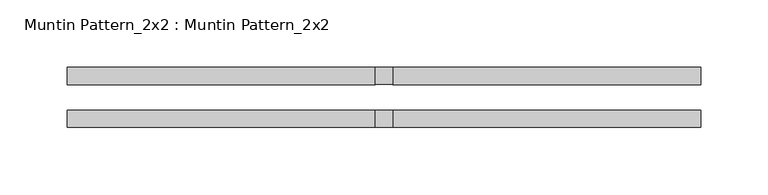
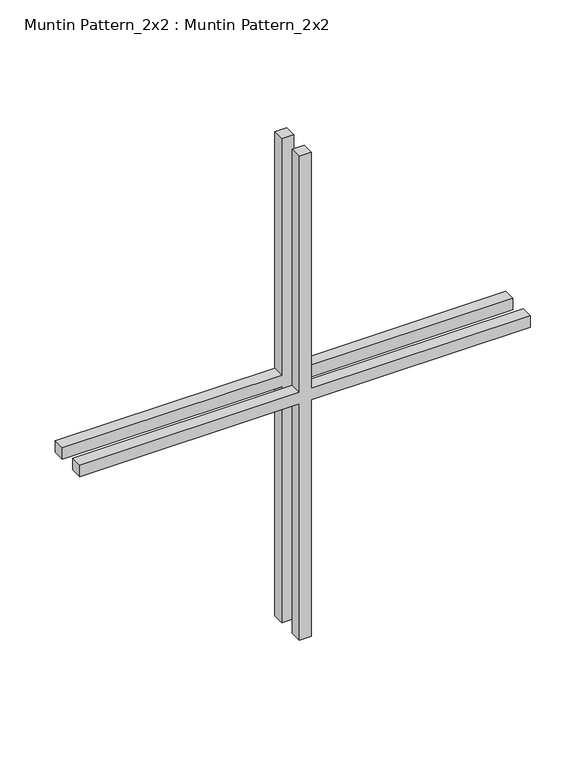
"""IFC4 building model written with IfcOpenShell, lengths in millimetres: proxy geometry, Muntin Pattern_2x2 : Muntin Pattern_2x2."""

from ifc_helpers import new_model, si_unit, frame, origin, place, context, project, spatial, polyline, outline, extrude, source, transform, mapped, element, save


def muntin_pattern_2x2_muntin_pattern_2x2_fa24e407(model_context):
    return source(origin(), model_context, "Body", "SweptSolid", [
        extrude(outline(polyline([(273.05, -6.35), (273.05, -234.95), (260.35, -234.95), (260.35, -6.35), (0.0, -6.35), (0.0, 6.35), (260.35, 6.35), (260.35, 234.95), (273.05, 234.95), (273.05, 6.35), (533.4, 6.35), (533.4, -6.35), (273.05, -6.35)])), frame((0.0, -22.225, 0.0), z_axis=(0.0, 1.0, 0.0), x_axis=(0.0, 0.0, 1.0)), (0.0, 0.0, 1.0), 12.7),
        extrude(outline(polyline([(273.05, -6.35), (273.05, -234.95), (260.35, -234.95), (260.35, -6.35), (0.0, -6.35), (0.0, 6.35), (260.35, 6.35), (260.35, 234.95), (273.05, 234.95), (273.05, 6.35), (533.4, 6.35), (533.4, -6.35), (273.05, -6.35)])), frame((0.0, 9.525, 0.0), z_axis=(0.0, 1.0, 0.0), x_axis=(0.0, 0.0, 1.0)), (0.0, 0.0, 1.0), 12.7),
    ])


if __name__ == "__main__":
    model = new_model("IFC4")
    model_context = context("Model", 3, world=origin())
    ifc_project = project(units=[si_unit("LENGTHUNIT", "METRE", prefix="MILLI")], contexts=[model_context])
    site = spatial("IfcSite", under=ifc_project)
    building = spatial("IfcBuilding", under=site)
    placement = place(None, origin())
    muntin_pattern_2x2_muntin_pattern_2x2_shape = muntin_pattern_2x2_muntin_pattern_2x2_fa24e407(model_context)
    element("IfcBuildingElementProxy", 1, Name="Muntin Pattern_2x2 : Muntin Pattern_2x2", ObjectType="Muntin Pattern_2x2 : Muntin Pattern_2x2", at=placement, inside=building, context=model_context, shape_type="MappedRepresentation", body=[
        mapped(muntin_pattern_2x2_muntin_pattern_2x2_shape, transform((0.0, 0.0, 0.0), x_axis=(1.0, 0.0, 0.0), y_axis=(0.0, 1.0, 0.0), z_axis=(0.0, 0.0, 1.0))),
    ])
    save(model, "model.ifc")

# Revit data of these elements
# Type "Muntin Pattern_2x2 : Muntin Pattern_2x2"
#   Width [instance default] = 4' - 0"
#   Thickness = 0' - 0 1/2"
#   Height [instance default] = 4' - 0"
#   Distance = 0' - 0 3/4"
#   Interior Material [instance default] = none
#   Exterior Material [instance default] = none
#   Default Elevation = 0
# Element 1 (IfcBuildingElementProxy, "Muntin Pattern_2x2 : Muntin Pattern_2x2")
#   Width = 1' - 6 1/2"
#   Height = 1' - 9"
#   Interior Material = Wood - Stained
#   Exterior Material = Clad - White
#   Materials on its faces: "Clad - White", "Wood - Stained"
# Materials
#   "Clad - White": class "Wood", colour RGB 242 242 238, transparency 0, Cost = 0
#   "Wood - Stained": class "Wood", colour RGB 224 178 126, transparency 0, Cost = 0
